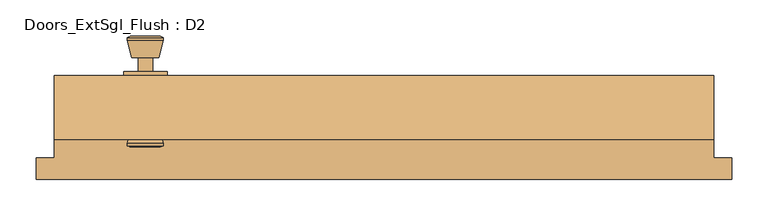
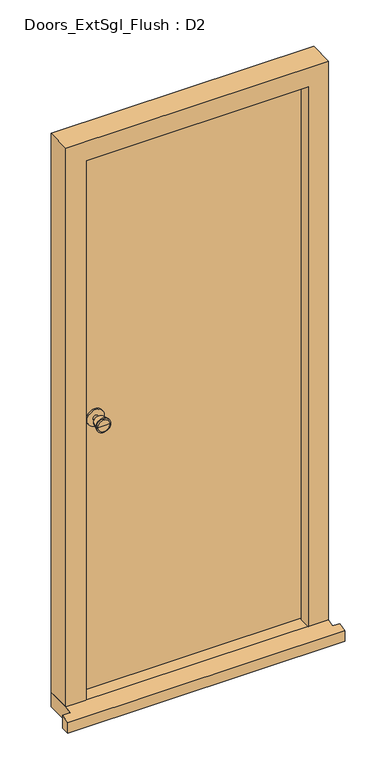
"""IFC4 building model written with IfcOpenShell, lengths in millimetres: door geometry, Doors_ExtSgl_Flush : D2."""

from ifc_helpers import new_model, si_unit, point, frame, frame_2d, origin, place, context, project, spatial, polyline, circle_curve, trimmed, segment, composite_curve, outline, extrude, faceted_brep, source, transform, mapped, element, save
from ifc_brep_helpers import plane_surface, cylinder_surface, revolved_surface, advanced_brep


def doors_extsgl_flush_d2_fac1298c(model_context):
    return source(origin(), model_context, "Body", "SolidModel", [
        advanced_brep(
        [(-330.7, 43.8, 1050.0), (-340.7, 43.8, 1050.0), (-320.7, 43.8, 1050.0), (-310.2241324, 92.8, 1050.0), (-351.1758676, 92.8, 1050.0), (-330.7, 92.8, 1050.0), (-305.7, 90.9721319, 1050.0), (-355.7, 90.9721319, 1050.0), (-305.7, 87.5084537, 1050.0), (-355.7, 87.5084537, 1050.0), (-312.063764, 62.8, 1050.0), (-349.336236, 62.8, 1050.0), (-320.7, 62.8, 1050.0), (-340.7, 62.8, 1050.0)],
        [
            (0, 1),
            (1, 2, circle_curve(frame((-330.7, 43.8, 1050.0), z_axis=(0.0, -1.0, 0.0), x_axis=(-1.0, 0.0, 0.0)), 10.0)),
            (2, 0),
            (2, 1, circle_curve(frame((-330.7, 43.8, 1050.0), z_axis=(0.0, -1.0, 0.0), x_axis=(-1.0, 0.0, 0.0)), 10.0)),
            (3, 4, circle_curve(frame((-330.7, 92.8, 1050.0), z_axis=(0.0, 1.0, 0.0), x_axis=(-1.0, 0.0, 0.0)), 20.4758676)),
            (4, 5),
            (5, 3),
            (4, 3, circle_curve(frame((-330.7, 92.8, 1050.0), z_axis=(0.0, 1.0, 0.0), x_axis=(-1.0, 0.0, 0.0)), 20.4758676)),
            (6, 7, circle_curve(frame((-330.7, 90.9721319, 1050.0), z_axis=(0.0, 1.0, 0.0), x_axis=(-1.0, 0.0, 0.0)), 25.0)),
            (7, 4),
            (3, 6),
            (7, 6, circle_curve(frame((-330.7, 90.9721319, 1050.0), z_axis=(0.0, 1.0, 0.0), x_axis=(-1.0, 0.0, 0.0)), 25.0)),
            (8, 9, circle_curve(frame((-330.7, 87.5084537, 1050.0), z_axis=(0.0, 1.0, 0.0), x_axis=(-1.0, 0.0, 0.0)), 25.0)),
            (9, 7),
            (6, 8),
            (9, 8, circle_curve(frame((-330.7, 87.5084537, 1050.0), z_axis=(0.0, 1.0, 0.0), x_axis=(-1.0, 0.0, 0.0)), 25.0)),
            (10, 11, circle_curve(frame((-330.7, 62.8, 1050.0), z_axis=(0.0, 1.0, 0.0), x_axis=(-1.0, 0.0, 0.0)), 18.636236)),
            (11, 9),
            (8, 10),
            (11, 10, circle_curve(frame((-330.7, 62.8, 1050.0), z_axis=(0.0, 1.0, 0.0), x_axis=(-1.0, 0.0, 0.0)), 18.636236)),
            (12, 13, circle_curve(frame((-330.7, 62.8, 1050.0), z_axis=(0.0, 1.0, 0.0), x_axis=(-1.0, 0.0, 0.0)), 10.0)),
            (13, 11),
            (10, 12),
            (13, 12, circle_curve(frame((-330.7, 62.8, 1050.0), z_axis=(0.0, 1.0, 0.0), x_axis=(-1.0, 0.0, 0.0)), 10.0)),
            (1, 13),
            (12, 2),
        ],
        [
            plane_surface(frame((-330.7, 43.8, 1050.0), z_axis=(0.0, -1.0, 0.0), x_axis=(-1.0, 0.0, 0.0))),
            plane_surface(frame((-330.7, 92.8, 1050.0), z_axis=(0.0, 1.0, 0.0), x_axis=(-1.0, 0.0, 0.0))),
            revolved_surface(polyline([(-351.1758676, 92.8, 1050.0), (-355.7, 90.9721319, 1050.0)]), (-330.7, 43.8, 1050.0), (0.0, -1.0, 0.0)),
            cylinder_surface(frame((-330.7, 43.8, 1050.0), z_axis=(0.0, -1.0, 0.0), x_axis=(-1.0, 0.0, 0.0)), 25.0),
            revolved_surface(polyline([(-355.7, 87.5084537, 1050.0), (-349.336236, 62.8, 1050.0)]), (-330.7, 43.8, 1050.0), (0.0, -1.0, 0.0)),
            plane_surface(frame((-330.7, 62.8, 1050.0), z_axis=(0.0, -1.0, 0.0), x_axis=(-1.0, 0.0, 0.0))),
            cylinder_surface(frame((-330.7, 43.8, 1050.0), z_axis=(0.0, -1.0, 0.0), x_axis=(-1.0, 0.0, 0.0)), 10.0),
        ],
        [
            (0, [[1, 2, 3]]),
            (0, [[-3, 4, -1]]),
            (1, [[5, 6, 7]]),
            (1, [[8, -7, -6]]),
            (2, [[9, 10, -5, 11]]),
            (2, [[12, -11, -8, -10]]),
            (3, [[13, 14, -9, 15]]),
            (3, [[16, -15, -12, -14]]),
            (4, [[17, 18, -13, 19]]),
            (4, [[20, -19, -16, -18]]),
            (5, [[21, 22, -17, 23]]),
            (5, [[24, -23, -20, -22]]),
            (6, [[-2, 25, -21, 26]]),
            (6, [[-4, -26, -24, -25]]),
        ],
    ),
        extrude(outline(composite_curve([segment(trimmed(circle_curve(frame_2d((1050.0, -330.7)), 30.0), [point((1050.0, -360.7))], [point((1050.0, -300.7))], False, "CARTESIAN"), True, "CONTINUOUS"), segment(trimmed(circle_curve(frame_2d((1050.0, -330.7)), 30.0), [point((1050.0, -300.7))], [point((1050.0, -360.7))], False, "CARTESIAN"), True, "CONTINUOUS")], self_intersect=False)), frame((0.0, 37.8, 0.0), z_axis=(0.0, 1.0, 0.0), x_axis=(0.0, 0.0, 1.0)), (0.0, 0.0, 1.0), 6.0),
        advanced_brep(
        [(-330.7, -12.2, 1050.0), (-320.7, -12.2, 1050.0), (-340.7, -12.2, 1050.0), (-310.2241324, -61.2, 1050.0), (-330.7, -61.2, 1050.0), (-351.1758676, -61.2, 1050.0), (-305.7, -59.3721319, 1050.0), (-355.7, -59.3721319, 1050.0), (-305.7, -55.9084537, 1050.0), (-355.7, -55.9084537, 1050.0), (-312.063764, -31.2, 1050.0), (-349.336236, -31.2, 1050.0), (-320.7, -31.2, 1050.0), (-340.7, -31.2, 1050.0)],
        [
            (0, 1),
            (1, 2, circle_curve(frame((-330.7, -12.2, 1050.0), z_axis=(0.0, 1.0, 0.0), x_axis=(-1.0, 0.0, 0.0)), 10.0)),
            (2, 0),
            (2, 1, circle_curve(frame((-330.7, -12.2, 1050.0), z_axis=(0.0, 1.0, 0.0), x_axis=(-1.0, 0.0, 0.0)), 10.0)),
            (3, 4),
            (4, 5),
            (5, 3, circle_curve(frame((-330.7, -61.2, 1050.0), z_axis=(0.0, -1.0, 0.0), x_axis=(-1.0, 0.0, 0.0)), 20.4758676)),
            (3, 5, circle_curve(frame((-330.7, -61.2, 1050.0), z_axis=(0.0, -1.0, 0.0), x_axis=(-1.0, 0.0, 0.0)), 20.4758676)),
            (6, 3),
            (5, 7),
            (7, 6, circle_curve(frame((-330.7, -59.3721319, 1050.0), z_axis=(0.0, -1.0, 0.0), x_axis=(-1.0, 0.0, 0.0)), 25.0)),
            (6, 7, circle_curve(frame((-330.7, -59.3721319, 1050.0), z_axis=(0.0, -1.0, 0.0), x_axis=(-1.0, 0.0, 0.0)), 25.0)),
            (8, 6),
            (7, 9),
            (9, 8, circle_curve(frame((-330.7, -55.9084537, 1050.0), z_axis=(0.0, -1.0, 0.0), x_axis=(-1.0, 0.0, 0.0)), 25.0)),
            (8, 9, circle_curve(frame((-330.7, -55.9084537, 1050.0), z_axis=(0.0, -1.0, 0.0), x_axis=(-1.0, 0.0, 0.0)), 25.0)),
            (10, 8),
            (9, 11),
            (11, 10, circle_curve(frame((-330.7, -31.2, 1050.0), z_axis=(0.0, -1.0, 0.0), x_axis=(-1.0, 0.0, 0.0)), 18.636236)),
            (10, 11, circle_curve(frame((-330.7, -31.2, 1050.0), z_axis=(0.0, -1.0, 0.0), x_axis=(-1.0, 0.0, 0.0)), 18.636236)),
            (12, 10),
            (11, 13),
            (13, 12, circle_curve(frame((-330.7, -31.2, 1050.0), z_axis=(0.0, -1.0, 0.0), x_axis=(-1.0, 0.0, 0.0)), 10.0)),
            (12, 13, circle_curve(frame((-330.7, -31.2, 1050.0), z_axis=(0.0, -1.0, 0.0), x_axis=(-1.0, 0.0, 0.0)), 10.0)),
            (1, 12),
            (13, 2),
        ],
        [
            plane_surface(frame((-330.7, -12.2, 1050.0), z_axis=(0.0, 1.0, 0.0), x_axis=(-1.0, 0.0, 0.0))),
            plane_surface(frame((-330.7, -61.2, 1050.0), z_axis=(0.0, -1.0, 0.0), x_axis=(-1.0, 0.0, 0.0))),
            revolved_surface(polyline([(-351.1758676, -61.2, 1050.0), (-355.7, -59.3721319, 1050.0)]), (-330.7, -12.2, 1050.0), (0.0, 1.0, 0.0)),
            cylinder_surface(frame((-330.7, -12.2, 1050.0), z_axis=(0.0, 1.0, 0.0), x_axis=(-1.0, 0.0, 0.0)), 25.0),
            revolved_surface(polyline([(-355.7, -55.9084537, 1050.0), (-349.336236, -31.2, 1050.0)]), (-330.7, -12.2, 1050.0), (0.0, 1.0, 0.0)),
            plane_surface(frame((-330.7, -31.2, 1050.0), z_axis=(0.0, 1.0, 0.0), x_axis=(-1.0, 0.0, 0.0))),
            cylinder_surface(frame((-330.7, -12.2, 1050.0), z_axis=(0.0, 1.0, 0.0), x_axis=(-1.0, 0.0, 0.0)), 10.0),
        ],
        [
            (0, [[1, 2, 3]]),
            (0, [[-3, 4, -1]]),
            (1, [[5, 6, 7]]),
            (1, [[-6, -5, 8]]),
            (2, [[9, -7, 10, 11]]),
            (2, [[-10, -8, -9, 12]]),
            (3, [[13, -11, 14, 15]]),
            (3, [[-14, -12, -13, 16]]),
            (4, [[17, -15, 18, 19]]),
            (4, [[-18, -16, -17, 20]]),
            (5, [[21, -19, 22, 23]]),
            (5, [[-22, -20, -21, 24]]),
            (6, [[25, -23, 26, -2]]),
            (6, [[-26, -24, -25, -4]]),
        ],
    ),
        extrude(outline(composite_curve([segment(trimmed(circle_curve(frame_2d((1050.0, -330.7)), 30.0), [point((1050.0, -360.7))], [point((1050.0, -300.7))], False, "CARTESIAN"), True, "CONTINUOUS"), segment(trimmed(circle_curve(frame_2d((1050.0, -330.7)), 30.0), [point((1050.0, -300.7))], [point((1050.0, -360.7))], False, "CARTESIAN"), True, "CONTINUOUS")], self_intersect=False)), frame((0.0, -12.2, 0.0), z_axis=(0.0, 1.0, 0.0), x_axis=(0.0, 0.0, 1.0)), (0.0, 0.0, 1.0), 6.0),
        faceted_brep([(386.7, -51.2, 54.5), (386.7, -9.2, 54.5), (408.7, -9.2, 54.5), (408.7, 37.8, 54.5), (457.2, 37.8, 54.5), (457.2, -51.2, 54.5), (457.2, -51.2, 2110.0), (-457.2, -51.2, 2110.0), (-457.2, -51.2, 54.5), (-386.7, -51.2, 54.5), (-386.7, -51.2, 2039.5), (386.7, -51.2, 2039.5), (457.2, 37.8, 2110.0), (408.7, 37.8, 2061.5), (-408.7, 37.8, 2061.5), (-408.7, 37.8, 54.5), (-457.2, 37.8, 54.5), (-457.2, 37.8, 2110.0), (408.7, -9.2, 2061.5), (386.7, -9.2, 2039.5), (-386.7, -9.2, 2039.5), (-386.7, -9.2, 54.5), (-408.7, -9.2, 54.5), (-408.7, -9.2, 2061.5)], [[[0, 1, 2, 3, 4, 5]], [[5, 6, 7, 8, 9, 10, 11, 0]], [[4, 12, 6, 5]], [[3, 13, 14, 15, 16, 17, 12, 4]], [[2, 18, 13, 3]], [[1, 19, 20, 21, 22, 23, 18, 2]], [[0, 11, 19, 1]], [[10, 9, 21, 20]], [[9, 8, 16, 15, 22, 21]], [[17, 16, 8, 7]], [[23, 22, 15, 14]], [[12, 17, 7, 6]], [[18, 23, 14, 13]], [[11, 10, 20, 19]]]),
        extrude(outline(polyline([(405.7, 37.8), (405.7, -6.2), (-406.6250294, -6.2), (-406.6250294, 37.8), (405.7, 37.8)])), frame((0.0, 0.0, 58.5), z_axis=(0.0, 0.0, 1.0), x_axis=(1.0, 0.0, 0.0)), (0.0, 0.0, 1.0), 2000.0),
        faceted_brep([(482.2, -106.2, 0.0), (482.2, -76.2, 0.0), (482.2, -76.2, 47.2703282), (482.2, -106.2, 38.5947221), (-482.2, -106.2, 38.5947221), (-482.2, -76.2, 47.2703282), (-482.2, -76.2, 0.0), (-482.2, -106.2, 0.0), (-457.2, -76.2, 0.0), (-457.2, 37.8, 0.0), (457.2, 37.8, 0.0), (457.2, -76.2, 0.0), (457.2, -76.2, 47.2703282), (457.2, -51.2, 54.5), (-457.2, -51.2, 54.5), (-457.2, -76.2, 47.2703282), (457.2, 37.8, 54.5), (-457.2, 37.8, 54.5)], [[[0, 1, 2, 3]], [[4, 5, 6, 7]], [[7, 6, 8, 9, 10, 11, 1, 0]], [[3, 4, 7, 0]], [[3, 2, 12, 13, 14, 15, 5, 4]], [[14, 13, 16, 17]], [[17, 16, 10, 9]], [[15, 14, 17, 9, 8]], [[8, 6, 5, 15]], [[11, 10, 16, 13, 12]], [[12, 2, 1, 11]]]),
    ])


if __name__ == "__main__":
    model = new_model("IFC4")
    model_context = context("Model", 3, world=origin())
    ifc_project = project(units=[si_unit("LENGTHUNIT", "METRE", prefix="MILLI")], contexts=[model_context])
    site = spatial("IfcSite", under=ifc_project)
    building = spatial("IfcBuilding", under=site)
    placement = place(None, origin())
    doors_extsgl_flush_d2_shape = doors_extsgl_flush_d2_fac1298c(model_context)
    element("IfcDoor", 1, ObjectType="Doors_ExtSgl_Flush : D2", at=placement, inside=building, context=model_context, shape_type="MappedRepresentation", body=[
        mapped(doors_extsgl_flush_d2_shape, transform((0.0, 0.0, 0.0), x_axis=(1.0, 0.0, 0.0), y_axis=(0.0, 1.0, 0.0), z_axis=(0.0, 0.0, 1.0))),
    ])
    save(model, "model.ifc")

# Revit data of these elements
# Type "Doors_ExtSgl_Flush : D2"
#   Type Mark = "50"
#   Type Comments = "External Single"
#   Operation = "SingleSwingRight"
#   Construction Type Id = "MDOOR"
#   Keynote = "L20"
#   Analytic Construction = "Metal"
#   Wrap Layers (Int) from Ext = 177.5 mm
#   Wrap Layers (Ext) from Ext = 102.5 mm
#   Thickness = 44 mm
#   Rough Width = 914.4 mm
#   Rough Height = 2110 mm
#   O/A Frame Width = 64 mm
#   Heat Transfer Coefficient (U) = 3.7021 W/(m²·K)
#   Handle Z Distance = 1050 mm
#   FrameWidth = 42 mm
#   FrameOffset - External = 25 mm
#   FrameDepth = 89 mm
#   Door Panel Width = 811.4 mm
#   Door Panel Thickness = 44 mm
#   Door Panel Height = 2000 mm
#   Cill Thickness = 54.5 mm
#   Cill Projection = 30 mm
#   Handle X Distance = 75 mm
#   Height = 2110 mm
#   Structural Tolerance = 6.5 mm
#   Tolerance = 3 mm
#   Undercut = 4 mm
#   Width = 914.4 mm
#   Cill Extension = 25 mm
#   Cavity Closer Width = 50 mm
#   Cavity Closer Offset from Ext = 102.5 mm
#   Cavity Closer Depth = 85 mm
#   Vis - Ironmongery = yes
#   Vis - Cavity Closers = yes
#   Define Thermal Properties by = 1
#   Function = 1
#   Material Door = Door - Panel
#   Material Frame = Door - Frame/Mullion
#   Material Ironmongery = Door - Handle
#   Visual Light Transmittance = 0
#   Solar Heat Gain Coefficient = 0
#   Wall Closure = (empty or 0)
# Element 1 (IfcDoor, "Doors_ExtSgl_Flush : D2")
#   Materials on its faces: "Door - Handle", "Door - Frame/Mullion", "Door - Panel"
# Materials
#   "Door - Panel": class "Wood", colour RGB 210 159 95, transparency 0, Keynote = "L20", Cost = 0
#   "Door - Frame/Mullion": class "Wood", colour RGB 212 179 113, transparency 0, Keynote = "L20", Cost = 0
#   "Door - Handle": colour RGB 0 0 0, transparency 0, Keynote = "P21", Cost = 0
